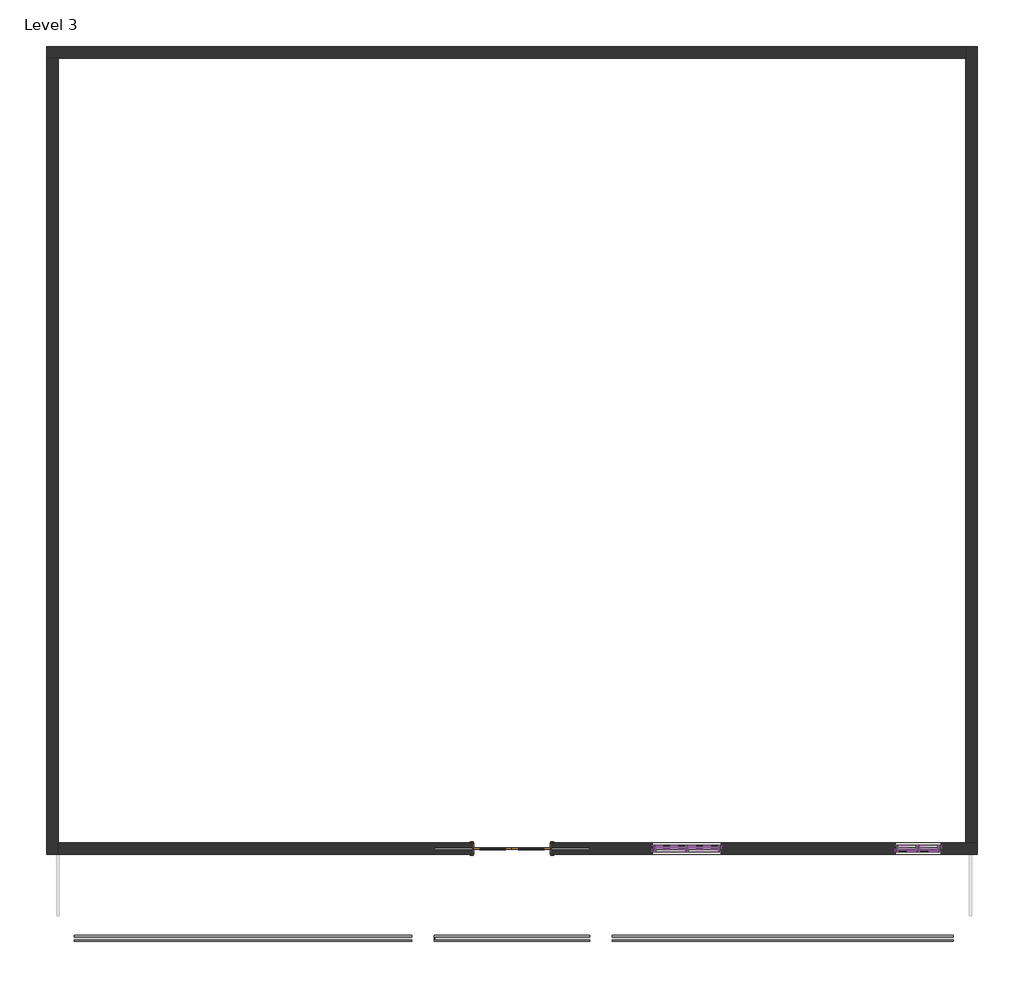
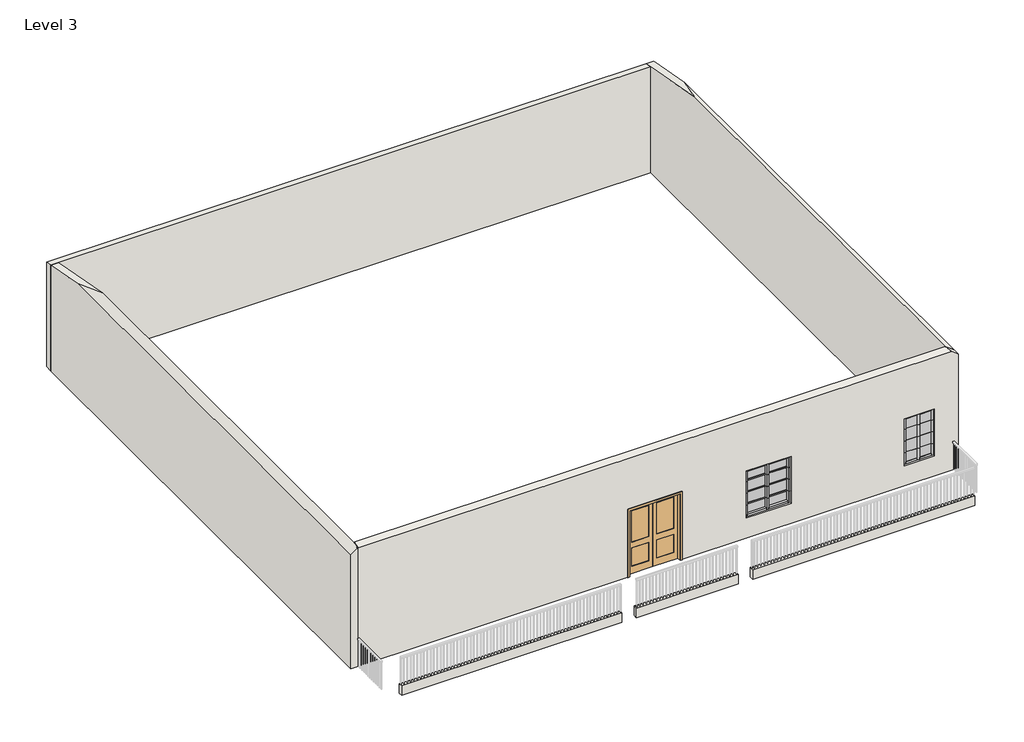
# One storey, part 1 of 3: 44 members, 16 plates, 7 walls, 1 door.
"""IFC4 building model written with IfcOpenShell, lengths in millimetres."""

from ifc_helpers import new_model, si_unit, frame, origin, place, context, project, spatial, polyline, outline, extrude, faceted_brep, transform, mapped, element, save
from components import door_7a66d0d1, member_2344d604, member_c698ba88, member_03a502dc, member_dfe75557, member_843225dc, member_e5d39754, member_76ae402a, member_f0218dda, system_panel_glazed_c76c6b52, system_panel_glazed_5d34ab6a, system_panel_glazed_40061ca4, system_panel_glazed_dbf5bbc8, system_panel_glazed_fa889304, system_panel_glazed_bcdea059

model = new_model("IFC4")

# Units and contexts
model_context = context("Model", 3, world=origin())
ifc_project = project(units=[si_unit("LENGTHUNIT", "METRE", prefix="MILLI")], contexts=[model_context])

# Site, building, storey
site = spatial("IfcSite", under=ifc_project)
building = spatial("IfcBuilding", under=site)
storey = spatial("IfcBuildingStorey", under=building, Name="Level 3", Elevation=3810.0)

# Door
placement = place(None, origin())
door_shape = door_7a66d0d1(model_context)
element("IfcDoor", 1, ObjectType="Door-Interior-Double-Pocket-2_Panel-Wood : 60\" x 84\"", at=placement, inside=storey, context=model_context, shape_type="MappedRepresentation", body=[
    mapped(door_shape, transform((-512.1420659, -6986.1878342, 3810.0), x_axis=(1.0, 0.0, 0.0), y_axis=(0.0, 1.0, 0.0), z_axis=(0.0, 0.0, 1.0))),
])

# Members
member_shape = member_2344d604(model_context)
element("IfcMember", 2, ObjectType="Rectangular Mullion : 1\" Square", at=placement, inside=storey, context=model_context, shape_type="MappedRepresentation", body=[
    mapped(member_shape, transform((7171.3579341, -6986.1878342, 5588.0), x_axis=(0.0, 0.0, 1.0), y_axis=(0.0, 1.0, 0.0), z_axis=(-1.0, 0.0, 0.0))),
])
element("IfcMember", 3, ObjectType="Rectangular Mullion : 1\" Square", at=placement, inside=storey, context=model_context, shape_type="MappedRepresentation", body=[
    mapped(member_shape, transform((7596.8079341, -6986.1878342, 5588.0), x_axis=(0.0, 0.0, 1.0), y_axis=(0.0, 1.0, 0.0), z_axis=(-1.0, 0.0, 0.0))),
])
element("IfcMember", 4, ObjectType="Rectangular Mullion : 1\" Square", at=placement, inside=storey, context=model_context, shape_type="MappedRepresentation", body=[
    mapped(member_shape, transform((7171.3579341, -6986.1878342, 5207.0), x_axis=(0.0, 0.0, 1.0), y_axis=(0.0, 1.0, 0.0), z_axis=(-1.0, 0.0, 0.0))),
])
element("IfcMember", 5, ObjectType="Rectangular Mullion : 1\" Square", at=placement, inside=storey, context=model_context, shape_type="MappedRepresentation", body=[
    mapped(member_shape, transform((7596.8079341, -6986.1878342, 5207.0), x_axis=(0.0, 0.0, 1.0), y_axis=(0.0, 1.0, 0.0), z_axis=(-1.0, 0.0, 0.0))),
])
element("IfcMember", 6, ObjectType="Rectangular Mullion : 1\" Square", at=placement, inside=storey, context=model_context, shape_type="MappedRepresentation", body=[
    mapped(member_shape, transform((7171.3579341, -6986.1878342, 4826.0), x_axis=(0.0, 0.0, 1.0), y_axis=(0.0, 1.0, 0.0), z_axis=(-1.0, 0.0, 0.0))),
])
element("IfcMember", 7, ObjectType="Rectangular Mullion : 1\" Square", at=placement, inside=storey, context=model_context, shape_type="MappedRepresentation", body=[
    mapped(member_shape, transform((7596.8079341, -6986.1878342, 4826.0), x_axis=(0.0, 0.0, 1.0), y_axis=(0.0, 1.0, 0.0), z_axis=(-1.0, 0.0, 0.0))),
])
member_2_shape = member_c698ba88(model_context)
element("IfcMember", 8, ObjectType="Rectangular Mullion : 1\" Square", at=placement, inside=storey, context=model_context, shape_type="MappedRepresentation", body=[
    mapped(member_2_shape, transform((3588.0949195, -6986.1878342, 5588.0), x_axis=(0.0, 0.0, 1.0), y_axis=(0.0, -1.0, 0.0), z_axis=(1.0, 0.0, 0.0))),
])
element("IfcMember", 9, ObjectType="Rectangular Mullion : 1\" Square", at=placement, inside=storey, context=model_context, shape_type="MappedRepresentation", body=[
    mapped(member_2_shape, transform((2934.0449195, -6986.1878342, 5588.0), x_axis=(0.0, 0.0, 1.0), y_axis=(0.0, -1.0, 0.0), z_axis=(1.0, 0.0, 0.0))),
])
element("IfcMember", 10, ObjectType="Rectangular Mullion : 1\" Square", at=placement, inside=storey, context=model_context, shape_type="MappedRepresentation", body=[
    mapped(member_2_shape, transform((3588.0949195, -6986.1878342, 5207.0), x_axis=(0.0, 0.0, 1.0), y_axis=(0.0, -1.0, 0.0), z_axis=(1.0, 0.0, 0.0))),
])
element("IfcMember", 11, ObjectType="Rectangular Mullion : 1\" Square", at=placement, inside=storey, context=model_context, shape_type="MappedRepresentation", body=[
    mapped(member_2_shape, transform((2934.0449195, -6986.1878342, 5207.0), x_axis=(0.0, 0.0, 1.0), y_axis=(0.0, -1.0, 0.0), z_axis=(1.0, 0.0, 0.0))),
])
element("IfcMember", 12, ObjectType="Rectangular Mullion : 1\" Square", at=placement, inside=storey, context=model_context, shape_type="MappedRepresentation", body=[
    mapped(member_2_shape, transform((3588.0949195, -6986.1878342, 4826.0), x_axis=(0.0, 0.0, 1.0), y_axis=(0.0, -1.0, 0.0), z_axis=(1.0, 0.0, 0.0))),
])
element("IfcMember", 13, ObjectType="Rectangular Mullion : 1\" Square", at=placement, inside=storey, context=model_context, shape_type="MappedRepresentation", body=[
    mapped(member_2_shape, transform((2934.0449195, -6986.1878342, 4826.0), x_axis=(0.0, 0.0, 1.0), y_axis=(0.0, -1.0, 0.0), z_axis=(1.0, 0.0, 0.0))),
])
member_3_shape = member_03a502dc(model_context)
element("IfcMember", 14, ObjectType="Rectangular Mullion : 2.5\" x 5\" rectangular", at=placement, inside=storey, context=model_context, shape_type="MappedRepresentation", body=[
    mapped(member_3_shape, transform((2965.7949195, -6986.1878342, 5588.0), x_axis=(1.0, 0.0, 0.0), y_axis=(0.0, -1.0, 0.0), z_axis=(0.0, 0.0, -1.0))),
])
element("IfcMember", 15, ObjectType="Rectangular Mullion : 2.5\" x 5\" rectangular", at=placement, inside=storey, context=model_context, shape_type="MappedRepresentation", body=[
    mapped(member_3_shape, transform((7565.0579341, -6986.1878342, 5588.0), x_axis=(-1.0, 0.0, 0.0), y_axis=(0.0, 1.0, 0.0), z_axis=(0.0, 0.0, -1.0))),
])
element("IfcMember", 16, ObjectType="Rectangular Mullion : 2.5\" x 5\" rectangular", at=placement, inside=storey, context=model_context, shape_type="MappedRepresentation", body=[
    mapped(member_3_shape, transform((2965.7949195, -6986.1878342, 5207.0), x_axis=(1.0, 0.0, 0.0), y_axis=(0.0, -1.0, 0.0), z_axis=(0.0, 0.0, -1.0))),
])
element("IfcMember", 17, ObjectType="Rectangular Mullion : 2.5\" x 5\" rectangular", at=placement, inside=storey, context=model_context, shape_type="MappedRepresentation", body=[
    mapped(member_3_shape, transform((2965.7949195, -6986.1878342, 4826.0), x_axis=(1.0, 0.0, 0.0), y_axis=(0.0, -1.0, 0.0), z_axis=(0.0, 0.0, -1.0))),
])
element("IfcMember", 18, ObjectType="Rectangular Mullion : 2.5\" x 5\" rectangular", at=placement, inside=storey, context=model_context, shape_type="MappedRepresentation", body=[
    mapped(member_3_shape, transform((7565.0579341, -6986.1878342, 5207.0), x_axis=(-1.0, 0.0, 0.0), y_axis=(0.0, 1.0, 0.0), z_axis=(0.0, 0.0, -1.0))),
])
element("IfcMember", 19, ObjectType="Rectangular Mullion : 2.5\" x 5\" rectangular", at=placement, inside=storey, context=model_context, shape_type="MappedRepresentation", body=[
    mapped(member_3_shape, transform((7565.0579341, -6986.1878342, 4826.0), x_axis=(-1.0, 0.0, 0.0), y_axis=(0.0, 1.0, 0.0), z_axis=(0.0, 0.0, -1.0))),
])
member_4_shape = member_dfe75557(model_context)
element("IfcMember", 20, ObjectType="Rectangular Mullion : 2.5\" x 5\" rectangular", at=placement, inside=storey, context=model_context, shape_type="MappedRepresentation", body=[
    mapped(member_4_shape, transform((2279.9949195, -6986.1878342, 5969.0), x_axis=(-1.0, 0.0, 0.0), y_axis=(0.0, -1.0, 0.0), z_axis=(0.0, 0.0, 1.0))),
])
element("IfcMember", 21, ObjectType="Rectangular Mullion : 2.5\" x 5\" rectangular", at=placement, inside=storey, context=model_context, shape_type="MappedRepresentation", body=[
    mapped(member_4_shape, transform((8022.2579341, -6986.1878342, 5969.0), x_axis=(1.0, 0.0, 0.0), y_axis=(0.0, 1.0, 0.0), z_axis=(0.0, 0.0, 1.0))),
])
element("IfcMember", 22, ObjectType="Rectangular Mullion : 2.5\" x 5\" rectangular", at=placement, inside=storey, context=model_context, shape_type="MappedRepresentation", body=[
    mapped(member_4_shape, transform((3651.5949195, -6986.1878342, 5588.0), x_axis=(1.0, 0.0, 0.0), y_axis=(0.0, -1.0, 0.0), z_axis=(0.0, 0.0, -1.0))),
])
element("IfcMember", 23, ObjectType="Rectangular Mullion : 2.5\" x 5\" rectangular", at=placement, inside=storey, context=model_context, shape_type="MappedRepresentation", body=[
    mapped(member_4_shape, transform((7107.8579341, -6986.1878342, 5588.0), x_axis=(-1.0, 0.0, 0.0), y_axis=(0.0, 1.0, 0.0), z_axis=(0.0, 0.0, -1.0))),
])
element("IfcMember", 24, ObjectType="Rectangular Mullion : 2.5\" x 5\" rectangular", at=placement, inside=storey, context=model_context, shape_type="MappedRepresentation", body=[
    mapped(member_4_shape, transform((3651.5949195, -6986.1878342, 5207.0), x_axis=(1.0, 0.0, 0.0), y_axis=(0.0, -1.0, 0.0), z_axis=(0.0, 0.0, -1.0))),
])
element("IfcMember", 25, ObjectType="Rectangular Mullion : 2.5\" x 5\" rectangular", at=placement, inside=storey, context=model_context, shape_type="MappedRepresentation", body=[
    mapped(member_4_shape, transform((3651.5949195, -6986.1878342, 4826.0), x_axis=(1.0, 0.0, 0.0), y_axis=(0.0, -1.0, 0.0), z_axis=(0.0, 0.0, -1.0))),
])
element("IfcMember", 26, ObjectType="Rectangular Mullion : 2.5\" x 5\" rectangular", at=placement, inside=storey, context=model_context, shape_type="MappedRepresentation", body=[
    mapped(member_4_shape, transform((7107.8579341, -6986.1878342, 5207.0), x_axis=(-1.0, 0.0, 0.0), y_axis=(0.0, 1.0, 0.0), z_axis=(0.0, 0.0, -1.0))),
])
element("IfcMember", 27, ObjectType="Rectangular Mullion : 2.5\" x 5\" rectangular", at=placement, inside=storey, context=model_context, shape_type="MappedRepresentation", body=[
    mapped(member_4_shape, transform((7107.8579341, -6986.1878342, 4826.0), x_axis=(-1.0, 0.0, 0.0), y_axis=(0.0, 1.0, 0.0), z_axis=(0.0, 0.0, -1.0))),
])
element("IfcMember", 28, ObjectType="Rectangular Mullion : 2.5\" x 5\" rectangular", at=placement, inside=storey, context=model_context, shape_type="MappedRepresentation", body=[
    mapped(member_4_shape, transform((2279.9949195, -6986.1878342, 5588.0), x_axis=(-1.0, 0.0, 0.0), y_axis=(0.0, -1.0, 0.0), z_axis=(0.0, 0.0, 1.0))),
])
element("IfcMember", 29, ObjectType="Rectangular Mullion : 2.5\" x 5\" rectangular", at=placement, inside=storey, context=model_context, shape_type="MappedRepresentation", body=[
    mapped(member_4_shape, transform((2279.9949195, -6986.1878342, 5207.0), x_axis=(-1.0, 0.0, 0.0), y_axis=(0.0, -1.0, 0.0), z_axis=(0.0, 0.0, 1.0))),
])
element("IfcMember", 30, ObjectType="Rectangular Mullion : 2.5\" x 5\" rectangular", at=placement, inside=storey, context=model_context, shape_type="MappedRepresentation", body=[
    mapped(member_4_shape, transform((8022.2579341, -6986.1878342, 5588.0), x_axis=(1.0, 0.0, 0.0), y_axis=(0.0, 1.0, 0.0), z_axis=(0.0, 0.0, 1.0))),
])
element("IfcMember", 31, ObjectType="Rectangular Mullion : 2.5\" x 5\" rectangular", at=placement, inside=storey, context=model_context, shape_type="MappedRepresentation", body=[
    mapped(member_4_shape, transform((8022.2579341, -6986.1878342, 5207.0), x_axis=(1.0, 0.0, 0.0), y_axis=(0.0, 1.0, 0.0), z_axis=(0.0, 0.0, 1.0))),
])
member_5_shape = member_843225dc(model_context)
element("IfcMember", 32, ObjectType="Rectangular Mullion : 2.5\" x 5\" rectangular", at=placement, inside=storey, context=model_context, shape_type="MappedRepresentation", body=[
    mapped(member_5_shape, transform((7958.7579341, -6986.1878342, 4454.4453853), x_axis=(0.0, 0.0, -1.0), y_axis=(0.0, 1.0, 0.0), z_axis=(1.0, 0.0, 0.0))),
])
element("IfcMember", 33, ObjectType="Rectangular Mullion : 2.5\" x 5\" rectangular", at=placement, inside=storey, context=model_context, shape_type="MappedRepresentation", body=[
    mapped(member_5_shape, transform((7533.3079341, -6986.1878342, 4454.4453853), x_axis=(0.0, 0.0, -1.0), y_axis=(0.0, 1.0, 0.0), z_axis=(1.0, 0.0, 0.0))),
])
element("IfcMember", 34, ObjectType="Rectangular Mullion : 2.5\" x 5\" rectangular", at=placement, inside=storey, context=model_context, shape_type="MappedRepresentation", body=[
    mapped(member_5_shape, transform((7171.3579341, -6986.1878342, 5969.0), x_axis=(0.0, 0.0, 1.0), y_axis=(0.0, 1.0, 0.0), z_axis=(-1.0, 0.0, 0.0))),
])
element("IfcMember", 35, ObjectType="Rectangular Mullion : 2.5\" x 5\" rectangular", at=placement, inside=storey, context=model_context, shape_type="MappedRepresentation", body=[
    mapped(member_5_shape, transform((7596.8079341, -6986.1878342, 5969.0), x_axis=(0.0, 0.0, 1.0), y_axis=(0.0, 1.0, 0.0), z_axis=(-1.0, 0.0, 0.0))),
])
member_6_shape = member_e5d39754(model_context)
element("IfcMember", 36, ObjectType="Rectangular Mullion : 2.5\" x 5\" rectangular", at=placement, inside=storey, context=model_context, shape_type="MappedRepresentation", body=[
    mapped(member_6_shape, transform((3588.0949195, -6986.1878342, 5969.0), x_axis=(0.0, 0.0, 1.0), y_axis=(0.0, -1.0, 0.0), z_axis=(1.0, 0.0, 0.0))),
])
element("IfcMember", 37, ObjectType="Rectangular Mullion : 2.5\" x 5\" rectangular", at=placement, inside=storey, context=model_context, shape_type="MappedRepresentation", body=[
    mapped(member_6_shape, transform((2934.0449195, -6986.1878342, 5969.0), x_axis=(0.0, 0.0, 1.0), y_axis=(0.0, -1.0, 0.0), z_axis=(1.0, 0.0, 0.0))),
])
element("IfcMember", 38, ObjectType="Rectangular Mullion : 2.5\" x 5\" rectangular", at=placement, inside=storey, context=model_context, shape_type="MappedRepresentation", body=[
    mapped(member_6_shape, transform((2343.4949195, -6986.1878342, 4454.4453853), x_axis=(0.0, 0.0, -1.0), y_axis=(0.0, -1.0, 0.0), z_axis=(-1.0, 0.0, 0.0))),
])
element("IfcMember", 39, ObjectType="Rectangular Mullion : 2.5\" x 5\" rectangular", at=placement, inside=storey, context=model_context, shape_type="MappedRepresentation", body=[
    mapped(member_6_shape, transform((2997.5449195, -6986.1878342, 4454.4453853), x_axis=(0.0, 0.0, -1.0), y_axis=(0.0, -1.0, 0.0), z_axis=(-1.0, 0.0, 0.0))),
])
member_7_shape = member_76ae402a(model_context)
element("IfcMember", 40, ObjectType="Rectangular Mullion : 2.5\" x 5\" rectangular", at=placement, inside=storey, context=model_context, shape_type="MappedRepresentation", body=[
    mapped(member_7_shape, transform((2965.7949195, -6986.1878342, 4454.4453853), x_axis=(1.0, 0.0, 0.0), y_axis=(0.0, -1.0, 0.0), z_axis=(0.0, 0.0, -1.0))),
])
element("IfcMember", 41, ObjectType="Rectangular Mullion : 2.5\" x 5\" rectangular", at=placement, inside=storey, context=model_context, shape_type="MappedRepresentation", body=[
    mapped(member_7_shape, transform((7565.0579341, -6986.1878342, 4454.4453853), x_axis=(-1.0, 0.0, 0.0), y_axis=(0.0, 1.0, 0.0), z_axis=(0.0, 0.0, -1.0))),
])
member_8_shape = member_f0218dda(model_context)
element("IfcMember", 42, ObjectType="Rectangular Mullion : 2.5\" x 5\" rectangular", at=placement, inside=storey, context=model_context, shape_type="MappedRepresentation", body=[
    mapped(member_8_shape, transform((3651.5949195, -6986.1878342, 4454.4453853), x_axis=(1.0, 0.0, 0.0), y_axis=(0.0, -1.0, 0.0), z_axis=(0.0, 0.0, -1.0))),
])
element("IfcMember", 43, ObjectType="Rectangular Mullion : 2.5\" x 5\" rectangular", at=placement, inside=storey, context=model_context, shape_type="MappedRepresentation", body=[
    mapped(member_8_shape, transform((7107.8579341, -6986.1878342, 4454.4453853), x_axis=(-1.0, 0.0, 0.0), y_axis=(0.0, 1.0, 0.0), z_axis=(0.0, 0.0, -1.0))),
])
element("IfcMember", 44, ObjectType="Rectangular Mullion : 2.5\" x 5\" rectangular", at=placement, inside=storey, context=model_context, shape_type="MappedRepresentation", body=[
    mapped(member_8_shape, transform((2279.9949195, -6986.1878342, 4826.0), x_axis=(-1.0, 0.0, 0.0), y_axis=(0.0, -1.0, 0.0), z_axis=(0.0, 0.0, 1.0))),
])
element("IfcMember", 45, ObjectType="Rectangular Mullion : 2.5\" x 5\" rectangular", at=placement, inside=storey, context=model_context, shape_type="MappedRepresentation", body=[
    mapped(member_8_shape, transform((8022.2579341, -6986.1878342, 4826.0), x_axis=(1.0, 0.0, 0.0), y_axis=(0.0, 1.0, 0.0), z_axis=(0.0, 0.0, 1.0))),
])

# Plates
system_panel_glazed_shape = system_panel_glazed_c76c6b52(model_context)
element("IfcPlate", 46, ObjectType="System Panel : Glazed", at=placement, inside=storey, context=model_context, shape_type="MappedRepresentation", body=[
    mapped(system_panel_glazed_shape, transform((7777.7829341, -6986.1878342, 5588.0), x_axis=(-1.0, 0.0, 0.0), y_axis=(0.0, -1.0, 0.0), z_axis=(0.0, 0.0, 1.0))),
])
element("IfcPlate", 47, ObjectType="System Panel : Glazed", at=placement, inside=storey, context=model_context, shape_type="MappedRepresentation", body=[
    mapped(system_panel_glazed_shape, transform((7352.3329341, -6986.1878342, 5588.0), x_axis=(-1.0, 0.0, 0.0), y_axis=(0.0, -1.0, 0.0), z_axis=(0.0, 0.0, 1.0))),
])
system_panel_glazed_2_shape = system_panel_glazed_5d34ab6a(model_context)
element("IfcPlate", 48, ObjectType="System Panel : Glazed", at=placement, inside=storey, context=model_context, shape_type="MappedRepresentation", body=[
    mapped(system_panel_glazed_2_shape, transform((7777.7829341, -6986.1878342, 5207.0), x_axis=(-1.0, 0.0, 0.0), y_axis=(0.0, -1.0, 0.0), z_axis=(0.0, 0.0, 1.0))),
])
element("IfcPlate", 49, ObjectType="System Panel : Glazed", at=placement, inside=storey, context=model_context, shape_type="MappedRepresentation", body=[
    mapped(system_panel_glazed_2_shape, transform((7352.3329341, -6986.1878342, 5207.0), x_axis=(-1.0, 0.0, 0.0), y_axis=(0.0, -1.0, 0.0), z_axis=(0.0, 0.0, 1.0))),
])
element("IfcPlate", 50, ObjectType="System Panel : Glazed", at=placement, inside=storey, context=model_context, shape_type="MappedRepresentation", body=[
    mapped(system_panel_glazed_2_shape, transform((7777.7829341, -6986.1878342, 4826.0), x_axis=(-1.0, 0.0, 0.0), y_axis=(0.0, -1.0, 0.0), z_axis=(0.0, 0.0, 1.0))),
])
element("IfcPlate", 51, ObjectType="System Panel : Glazed", at=placement, inside=storey, context=model_context, shape_type="MappedRepresentation", body=[
    mapped(system_panel_glazed_2_shape, transform((7352.3329341, -6986.1878342, 4826.0), x_axis=(-1.0, 0.0, 0.0), y_axis=(0.0, -1.0, 0.0), z_axis=(0.0, 0.0, 1.0))),
])
system_panel_glazed_3_shape = system_panel_glazed_40061ca4(model_context)
element("IfcPlate", 52, ObjectType="System Panel : Glazed", at=placement, inside=storey, context=model_context, shape_type="MappedRepresentation", body=[
    mapped(system_panel_glazed_3_shape, transform((2638.7699195, -6986.1878342, 4517.9453853), x_axis=(1.0, 0.0, 0.0), y_axis=(0.0, 1.0, 0.0), z_axis=(0.0, 0.0, 1.0))),
])
element("IfcPlate", 53, ObjectType="System Panel : Glazed", at=placement, inside=storey, context=model_context, shape_type="MappedRepresentation", body=[
    mapped(system_panel_glazed_3_shape, transform((3292.8199195, -6986.1878342, 4517.9453853), x_axis=(1.0, 0.0, 0.0), y_axis=(0.0, 1.0, 0.0), z_axis=(0.0, 0.0, 1.0))),
])
system_panel_glazed_4_shape = system_panel_glazed_dbf5bbc8(model_context)
element("IfcPlate", 54, ObjectType="System Panel : Glazed", at=placement, inside=storey, context=model_context, shape_type="MappedRepresentation", body=[
    mapped(system_panel_glazed_4_shape, transform((2638.7699195, -6986.1878342, 5588.0), x_axis=(1.0, 0.0, 0.0), y_axis=(0.0, 1.0, 0.0), z_axis=(0.0, 0.0, 1.0))),
])
element("IfcPlate", 55, ObjectType="System Panel : Glazed", at=placement, inside=storey, context=model_context, shape_type="MappedRepresentation", body=[
    mapped(system_panel_glazed_4_shape, transform((3292.8199195, -6986.1878342, 5588.0), x_axis=(1.0, 0.0, 0.0), y_axis=(0.0, 1.0, 0.0), z_axis=(0.0, 0.0, 1.0))),
])
system_panel_glazed_5_shape = system_panel_glazed_fa889304(model_context)
element("IfcPlate", 56, ObjectType="System Panel : Glazed", at=placement, inside=storey, context=model_context, shape_type="MappedRepresentation", body=[
    mapped(system_panel_glazed_5_shape, transform((2638.7699195, -6986.1878342, 5207.0), x_axis=(1.0, 0.0, 0.0), y_axis=(0.0, 1.0, 0.0), z_axis=(0.0, 0.0, 1.0))),
])
element("IfcPlate", 57, ObjectType="System Panel : Glazed", at=placement, inside=storey, context=model_context, shape_type="MappedRepresentation", body=[
    mapped(system_panel_glazed_5_shape, transform((3292.8199195, -6986.1878342, 5207.0), x_axis=(1.0, 0.0, 0.0), y_axis=(0.0, 1.0, 0.0), z_axis=(0.0, 0.0, 1.0))),
])
element("IfcPlate", 58, ObjectType="System Panel : Glazed", at=placement, inside=storey, context=model_context, shape_type="MappedRepresentation", body=[
    mapped(system_panel_glazed_5_shape, transform((2638.7699195, -6986.1878342, 4826.0), x_axis=(1.0, 0.0, 0.0), y_axis=(0.0, 1.0, 0.0), z_axis=(0.0, 0.0, 1.0))),
])
element("IfcPlate", 59, ObjectType="System Panel : Glazed", at=placement, inside=storey, context=model_context, shape_type="MappedRepresentation", body=[
    mapped(system_panel_glazed_5_shape, transform((3292.8199195, -6986.1878342, 4826.0), x_axis=(1.0, 0.0, 0.0), y_axis=(0.0, 1.0, 0.0), z_axis=(0.0, 0.0, 1.0))),
])
system_panel_glazed_6_shape = system_panel_glazed_bcdea059(model_context)
element("IfcPlate", 60, ObjectType="System Panel : Glazed", at=placement, inside=storey, context=model_context, shape_type="MappedRepresentation", body=[
    mapped(system_panel_glazed_6_shape, transform((7777.7829341, -6986.1878342, 4517.9453853), x_axis=(-1.0, 0.0, 0.0), y_axis=(0.0, -1.0, 0.0), z_axis=(0.0, 0.0, 1.0))),
])
element("IfcPlate", 61, ObjectType="System Panel : Glazed", at=placement, inside=storey, context=model_context, shape_type="MappedRepresentation", body=[
    mapped(system_panel_glazed_6_shape, transform((7352.3329341, -6986.1878342, 4517.9453853), x_axis=(-1.0, 0.0, 0.0), y_axis=(0.0, -1.0, 0.0), z_axis=(0.0, 0.0, 1.0))),
])

# Walls
element("IfcWall", 62, ObjectType="4.5\" wall", at=placement, inside=storey, context=model_context, shape_type="SweptSolid", body=[
    extrude(outline(polyline([(-2506.0420659, -8827.6878342), (-9224.3420659, -8827.6878342), (-9224.3420659, -8713.3878342), (-2506.0420659, -8713.3878342), (-2506.0420659, -8827.6878342)])), frame((0.0, 0.0, 3810.0), z_axis=(0.0, 0.0, 1.0), x_axis=(1.0, 0.0, 0.0)), (0.0, 0.0, 1.0), 304.8),
])
element("IfcWall", 63, ObjectType="4.5\" wall", at=placement, inside=storey, context=model_context, shape_type="SweptSolid", body=[
    extrude(outline(polyline([(1037.2579341, -8827.6878342), (-2061.5420659, -8827.6878342), (-2061.5420659, -8713.3878342), (1037.2579341, -8713.3878342), (1037.2579341, -8827.6878342)])), frame((0.0, 0.0, 3810.0), z_axis=(0.0, 0.0, 1.0), x_axis=(1.0, 0.0, 0.0)), (0.0, 0.0, 1.0), 304.8),
])
element("IfcWall", 64, ObjectType="4.5\" wall", at=placement, inside=storey, context=model_context, shape_type="SweptSolid", body=[
    extrude(outline(polyline([(8263.5579341, -8825.9902135), (1481.7579341, -8825.9902135), (1481.7579341, -8711.6902135), (8263.5579341, -8711.6902135), (8263.5579341, -8825.9902135)])), frame((0.0, 0.0, 3810.0), z_axis=(0.0, 0.0, 1.0), x_axis=(1.0, 0.0, 0.0)), (0.0, 0.0, 1.0), 304.8),
])
element("IfcWall", 65, ObjectType="9\" wall", at=placement, inside=storey, context=model_context, shape_type="Brep", body=[
    faceted_brep([(-9770.4420659, 8749.1121658, 3810.0), (-9541.8420659, 8749.1121658, 3810.0), (8517.5579341, 8749.1121658, 3810.0), (8517.5579341, 8749.1121658, 7218.0188309), (-9541.8420659, 8749.1121658, 7218.0188309), (-9770.4420659, 8749.1121658, 7218.0188309), (-9770.4420659, 8977.7121658, 3810.0), (-9770.4420659, 8977.7121658, 7175.2500589), (8517.5579341, 8977.7121658, 7175.2500589), (8517.5579341, 8977.7121658, 3810.0)], [[[0, 1, 2, 3, 4, 5]], [[6, 7, 8, 9]], [[2, 1, 0, 6, 9]], [[0, 5, 7, 6]], [[3, 2, 9, 8]], [[5, 4, 3, 8, 7]]]),
])
element("IfcWall", 66, ObjectType="9\" wall", at=placement, inside=storey, context=model_context, shape_type="Brep", body=[
    faceted_brep([(-9541.8420659, -7100.4878342, 3810.0), (-9541.8420659, -6871.8878342, 3810.0), (-9541.8420659, 8749.1121658, 3810.0), (-9541.8420659, 8749.1121658, 7218.0188309), (-9541.8420659, 6416.6761634, 7654.394263), (-9541.8420659, -6871.8878342, 7654.394263), (-9541.8420659, -6977.8518318, 7654.394263), (-9541.8420659, -7100.4878342, 7631.4502944), (-9770.4420659, -7100.4878342, 3810.0), (-9770.4420659, -7100.4878342, 7482.944263), (-9770.4420659, 7333.0800744, 7482.944263), (-9770.4420659, 8749.1121658, 7218.0188309), (-9770.4420659, 8749.1121658, 3810.0), (-9572.4340241, -7100.4878342, 7631.4502944)], [[[0, 1, 2, 3, 4, 5, 6, 7]], [[8, 9, 10, 11, 12]], [[2, 1, 0, 8, 12]], [[3, 2, 12, 11]], [[0, 7, 13, 9, 8]], [[4, 3, 11, 10]], [[7, 6, 13]], [[6, 5, 4, 10, 9, 13]]]),
])
element("IfcWall", 67, ObjectType="9\" wall", at=placement, inside=storey, context=model_context, shape_type="Brep", body=[
    faceted_brep([(8746.1579341, -6871.8878342, 7482.944263), (8746.1579341, -6871.8878342, 3810.0), (8517.5579341, -6871.8878342, 3810.0), (275.2579341, -6871.8878342, 3810.0), (275.2579341, -6871.8878342, 5969.0), (-1299.5420659, -6871.8878342, 5969.0), (-1299.5420659, -6871.8878342, 3810.0), (-9541.8420659, -6871.8878342, 3810.0), (-9541.8420659, -6871.8878342, 7654.394263), (-9515.4089947, -6871.8878342, 7674.2190664), (8491.1248629, -6871.8878342, 7674.2190664), (8517.5579341, -6871.8878342, 7654.394263), (2279.9949195, -6871.8878342, 5969.0), (2279.9949195, -6871.8878342, 4454.4453853), (3651.5949195, -6871.8878342, 4454.4453853), (3651.5949195, -6871.8878342, 5969.0), (8022.2579341, -6871.8878342, 4454.4453853), (8022.2579341, -6871.8878342, 5969.0), (7107.8579341, -6871.8878342, 5969.0), (7107.8579341, -6871.8878342, 4454.4453853), (8746.1579341, -7100.4878342, 3810.0), (8746.1579341, -7100.4878342, 7482.944263), (8548.1498923, -7100.4878342, 7631.4502944), (-9541.8420659, -7100.4878342, 7631.4502944), (-9541.8420659, -7100.4878342, 3810.0), (-1299.5420659, -7100.4878342, 3810.0), (-1299.5420659, -7100.4878342, 5969.0), (275.2579341, -7100.4878342, 5969.0), (275.2579341, -7100.4878342, 3810.0), (2279.9949195, -7100.4878342, 4454.4453853), (2279.9949195, -7100.4878342, 5969.0), (3651.5949195, -7100.4878342, 5969.0), (3651.5949195, -7100.4878342, 4454.4453853), (8022.2579341, -7100.4878342, 5969.0), (8022.2579341, -7100.4878342, 4454.4453853), (7107.8579341, -7100.4878342, 4454.4453853), (7107.8579341, -7100.4878342, 5969.0), (275.2579341, -7006.8253342, 3810.0), (1037.2579341, -7006.8253342, 3810.0), (1037.2579341, -6965.5503342, 3810.0), (275.2579341, -6965.5503342, 3810.0), (-1299.5420659, -6965.5503342, 3810.0), (-2061.5420659, -6965.5503342, 3810.0), (-2061.5420659, -7006.8253342, 3810.0), (-1299.5420659, -7006.8253342, 3810.0), (-9541.8420659, -6977.8518318, 7654.394263), (1037.2579341, -6965.5503342, 5969.0), (1037.2579341, -7006.8253342, 5969.0), (275.2579341, -7006.8253342, 5969.0), (-1299.5420659, -7006.8253342, 5969.0), (-2061.5420659, -7006.8253342, 5969.0), (-2061.5420659, -6965.5503342, 5969.0), (-1299.5420659, -6965.5503342, 5969.0), (275.2579341, -6965.5503342, 5969.0)], [[[0, 1, 2, 3, 4, 5, 6, 7, 8, 9, 10, 11], [12, 13, 14, 15], [16, 17, 18, 19]], [[20, 21, 22, 23, 24, 25, 26, 27, 28], [29, 30, 31, 32], [33, 34, 35, 36]], [[1, 20, 28, 37, 38, 39, 40, 3, 2]], [[24, 7, 6, 41, 42, 43, 44, 25]], [[1, 0, 21, 20]], [[8, 7, 24, 23, 45]], [[46, 47, 48, 27, 26, 49, 50, 51, 52, 5, 4, 53]], [[46, 53, 40, 39]], [[53, 4, 3, 40]], [[5, 52, 41, 6]], [[52, 51, 42, 41]], [[51, 50, 43, 42]], [[50, 49, 44, 43]], [[49, 26, 25, 44]], [[27, 48, 37, 28]], [[48, 47, 38, 37]], [[47, 46, 39, 38]], [[29, 13, 12, 30]], [[30, 12, 15, 31]], [[14, 32, 31, 15]], [[13, 29, 32, 14]], [[16, 34, 33, 17]], [[17, 33, 36, 18]], [[18, 36, 35, 19]], [[34, 16, 19, 35]], [[21, 0, 11, 10, 22]], [[10, 9, 45, 23, 22]], [[9, 8, 45]]]),
])
element("IfcWall", 68, ObjectType="9\" wall", at=placement, inside=storey, context=model_context, shape_type="Brep", body=[
    faceted_brep([(8517.5579341, 8977.7121658, 3810.0), (8517.5579341, 8749.1121658, 3810.0), (8517.5579341, -6871.8878342, 3810.0), (8517.5579341, -6871.8878342, 7654.394263), (8517.5579341, 6416.6761634, 7654.394263), (8517.5579341, 8749.1121658, 7218.0188309), (8517.5579341, 8977.7121658, 7175.2500589), (8746.1579341, 8977.7121658, 3810.0), (8746.1579341, 8977.7121658, 7175.2500589), (8746.1579341, 7333.0800744, 7482.944263), (8746.1579341, -6871.8878342, 7482.944263), (8746.1579341, -6871.8878342, 3810.0)], [[[0, 1, 2, 3, 4, 5, 6]], [[7, 8, 9, 10, 11]], [[2, 1, 0, 7, 11]], [[0, 6, 8, 7]], [[3, 2, 11, 10]], [[6, 5, 4, 9, 8]], [[4, 3, 10, 9]]]),
])

save(model, "model.ifc")

# Revit data of these elements
# Type "Door-Interior-Double-Pocket-2_Panel-Wood : 60\" x 84\""
#   Type Mark = "8"
#   Assembly Code = "C1020300"
#   Analytic Construction = "Wooden"
#   Top Rail = 0' - 4 11/16"
#   Thickness = 0' - 1 3/8"
#   Thermal Resistance (R) = 2.5876 (h·ft²·°F)/BTU
#   Stiles = 0' - 4 3/4"
#   Rough Width = 10' - 2"
#   Rough Height = 7' - 4 1/2"
#   Panel Width = 2' - 6"
#   Lock Rail = 0' - 7 1/2"
#   Location [instance default] = 2' - 7"
#   Height = 7' - 0"
#   Width = 5' - 0"
#   Heat Transfer Coefficient (U) = 0.3865 BTU/(h·ft²·°F)
#   Bottom Rail = 0' - 9 1/8"
#   Panel Open [instance default] = no
#   Trim Material = Cherry
#   Panel Material = Cherry
#   Frame Material = Cherry
#   Visual Light Transmittance = 0
#   Solar Heat Gain Coefficient = 0
#   Wall Closure = (empty or 0)
#   Function = (empty or 0)
# Type "Rectangular Mullion : 1\" Square"
#   built-in parameter 1007304 = 0.0833333 (stored number, unit not read)
#   built-in parameter 1007301 = 0.0416667 (stored number, unit not read)
#   built-in parameter 1007300 = 0.0416667 (stored number, unit not read)
# Type "Rectangular Mullion : 2.5\" x 5\" rectangular"
#   built-in parameter 1007304 = 0.416667 (stored number, unit not read)
#   built-in parameter 1007301 = 0.104167 (stored number, unit not read)
#   built-in parameter 1007300 = 0.104167 (stored number, unit not read)
# Type "System Panel : Glazed"
#   Construction Type Id = "GSP4R"
#   Analytic Construction = "1/8 in Pilkington single glazing"
#   Visual Light Transmittance = 0.9
#   Solar Heat Gain Coefficient = 0.86
#   Heat Transfer Coefficient (U) = 1.18115 BTU/(h·ft²·°F)
#   Define Thermal Properties by = 1
# Type "4.5\" wall"
#   Assembly Code = "B2010"
#   Layers, outside or top first: 0' - 4 1/2" "wood wall" (function 1)
# Type "9\" wall"
#   Assembly Code = "B2010"
# Element 1 (IfcDoor, "Door-Interior-Double-Pocket-2_Panel-Wood : 60\" x 84\"")
#   Location = 2' - 7"
#   Panel Open = no
#   Phase Created = New Construction
#   Materials on its faces: "Cherry"
# Elements 2, 3, 4, 5, 6, 7, 8, 9, 10, 11, 12, 13 (IfcMember, "Rectangular Mullion : 1\" Square")
#   Phase Created = New Construction
# Elements 14, 15, 16, 17, 18, 19, 20, 21, 22, 23, 24, 25, 26, 27, 28, 29, 30, 31, 32, 33, 34, 35, 36, 37, 38, 39, 40, 41, 42, 43, 44, 45 (IfcMember, "Rectangular Mullion : 2.5\" x 5\" rectangular")
#   Phase Created = New Construction
# Elements 46, 47, 48, 49, 50, 51, 52, 53, 54, 55, 56, 57, 58, 59, 60, 61 (IfcPlate, "System Panel : Glazed")
#   Phase Created = New Construction
#   Materials on its faces: "Glass"
# Elements 62, 63, 64 (IfcWall, "4.5\" wall")
#   Top Offset = -9' - 0"
#   Base Offset = 0' - 0"
#   wall height = 1' - 0"
#   Phase Created = New Construction
#   Base Constraint = Level 3
#   Top Constraint = Level 4
#   Materials on its faces: "wood wall"
# Elements 65, 66, 67, 68 (IfcWall, "9\" wall")
#   Top Offset = 1' - 6"
#   Base Offset = 0' - 0"
#   Unconnected Height = 12' - 0"
#   wall height = 12' - 0"
#   Phase Created = New Construction
#   Base Constraint = Level 3
# Materials
#   "Cherry": class "Wood", colour RGB 226 177 128, transparency 0, Description = "Prunus Serotina", Cost = 0
#   "wood wall": class "Generic", colour RGB 120 120 120, transparency 0, Cost = 0
#   "Glass": class "Glass", colour RGB 0 128 192, transparency 0.75, Description = "Soda Lime Glass", Cost = 0
